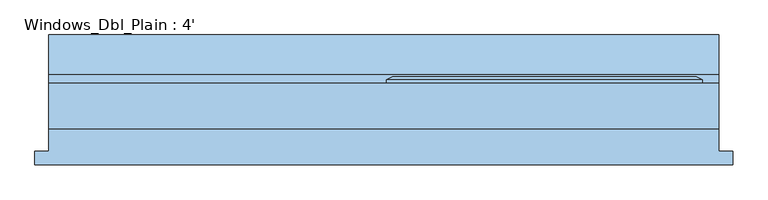
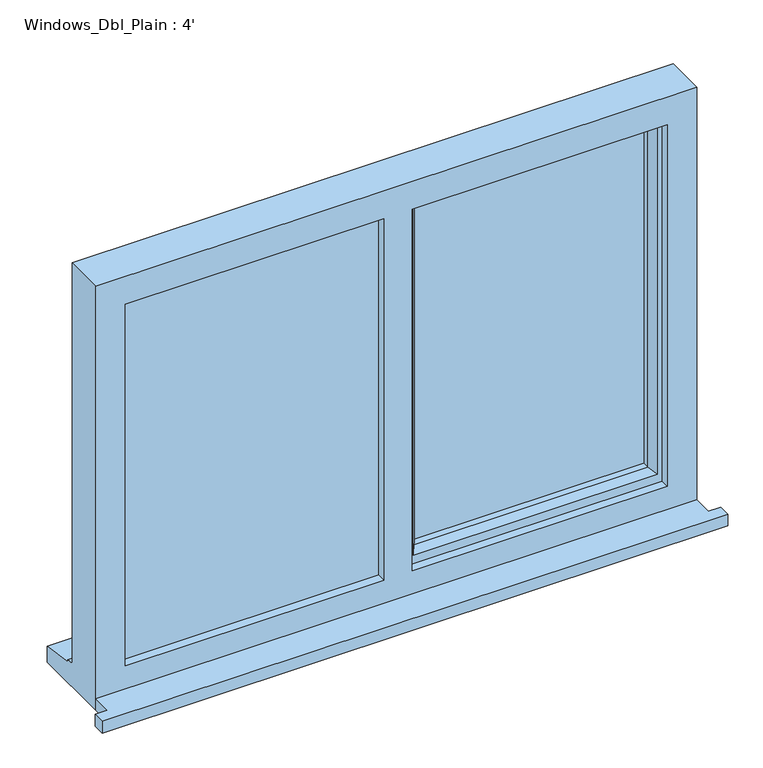
"""IFC4 building model written with IfcOpenShell, lengths in millimetres: window geometry, Windows_Dbl_Plain : 4'."""

from ifc_helpers import new_model, si_unit, frame, origin, place, context, project, spatial, polyline, outline, extrude, faceted_brep, source, transform, mapped, element, save


def windows_dbl_plain_4_44133fe2(model_context):
    return source(origin(), model_context, "Body", "SolidModel", [
        extrude(outline(polyline([(-919.6, -103.4114322), (-919.6, -78.4114322), (-894.6, -78.4114322), (-894.6, -37.6754322), (324.6, -37.6754322), (324.6, -78.4114322), (349.6, -78.4114322), (349.6, -103.4114322), (-919.6, -103.4114322)])), frame((0.0, 0.0, 1200.0), z_axis=(0.0, 0.0, 1.0), x_axis=(1.0, 0.0, 0.0)), (0.0, 0.0, 1.0), 25.0),
        faceted_brep([(-280.0, 45.3245678, 2080.0), (-280.0, 51.0980705, 2080.0), (-280.0, 51.0980705, 1253.0), (-280.0, 45.3245678, 1253.0), (-270.0, -19.6754322, 2070.0), (-270.0, 45.3245678, 2070.0), (-270.0, 45.3245678, 1263.0), (-270.0, -19.6754322, 1263.0), (-230.0, -5.1825323, 2030.0), (-240.1480377, -19.6754322, 2040.1480377), (-240.1480377, -19.6754322, 1292.8519623), (-230.0, -5.1825323, 1303.0), (-230.0, 9.3245678, 2030.0), (-230.0, 9.3245678, 1303.0), (-240.0, 33.3245678, 2040.0), (-240.0, 9.3245678, 2040.0), (-240.0, 9.3245678, 1293.0), (-240.0, 33.3245678, 1293.0), (-230.0, 51.0980705, 2030.0), (-230.0, 33.3245678, 2030.0), (-230.0, 33.3245678, 1303.0), (-230.0, 51.0980705, 1303.0), (-247.4457548, 56.8715732, 2047.4457548), (-247.4457548, 56.8715732, 1285.5542452), (-269.2153903, 56.8715732, 2069.2153903), (-269.2153903, 56.8715732, 1263.7846097), (294.6, 51.0980705, 1253.0), (294.6, 45.3245678, 1253.0), (284.6, 45.3245678, 1263.0), (284.6, -19.6754322, 1263.0), (254.7480377, -19.6754322, 1292.8519623), (244.6, -5.1825323, 1303.0), (244.6, 9.3245678, 1303.0), (254.6, 9.3245678, 1293.0), (254.6, 33.3245678, 1293.0), (244.6, 33.3245678, 1303.0), (244.6, 51.0980705, 1303.0), (262.0457548, 56.8715732, 1285.5542452), (283.8153903, 56.8715732, 1263.7846097), (294.6, 51.0980705, 2080.0), (294.6, 45.3245678, 2080.0), (284.6, 45.3245678, 2070.0), (284.6, -19.6754322, 2070.0), (254.7480377, -19.6754322, 2040.1480377), (244.6, -5.1825323, 2030.0), (244.6, 9.3245678, 2030.0), (254.6, 9.3245678, 2040.0), (254.6, 33.3245678, 2040.0), (244.6, 33.3245678, 2030.0), (244.6, 51.0980705, 2030.0), (262.0457548, 56.8715732, 2047.4457548), (283.8153903, 56.8715732, 2069.2153903)], [[[0, 1, 2, 3]], [[4, 5, 6, 7]], [[8, 9, 10, 11]], [[12, 8, 11, 13]], [[14, 15, 16, 17]], [[18, 19, 20, 21]], [[22, 18, 21, 23]], [[1, 24, 25, 2]], [[3, 2, 26, 27]], [[7, 6, 28, 29]], [[11, 10, 30, 31]], [[13, 11, 31, 32]], [[17, 16, 33, 34]], [[21, 20, 35, 36]], [[23, 21, 36, 37]], [[2, 25, 38, 26]], [[27, 26, 39, 40]], [[29, 28, 41, 42]], [[31, 30, 43, 44]], [[32, 31, 44, 45]], [[34, 33, 46, 47]], [[36, 35, 48, 49]], [[37, 36, 49, 50]], [[26, 38, 51, 39]], [[40, 39, 1, 0]], [[3, 27, 40, 0], [5, 41, 28, 6]], [[42, 41, 5, 4]], [[7, 29, 42, 4], [9, 43, 30, 10]], [[44, 43, 9, 8]], [[45, 44, 8, 12]], [[15, 46, 33, 16], [13, 32, 45, 12]], [[47, 46, 15, 14]], [[17, 34, 47, 14], [19, 48, 35, 20]], [[49, 48, 19, 18]], [[50, 49, 18, 22]], [[24, 51, 38, 25], [23, 37, 50, 22]], [[39, 51, 24, 1]]]),
        extrude(outline(polyline([(2050.0, -310.0), (2070.0, -310.0), (2070.0, -854.6), (1263.0, -854.6), (1263.0, -310.0), (1283.0, -310.0), (1283.0, -834.6), (2050.0, -834.6), (2050.0, -310.0)])), frame((0.0, 4.3245678, 0.0), z_axis=(0.0, 1.0, 0.0), x_axis=(0.0, 0.0, 1.0)), (0.0, 0.0, 1.0), 41.0),
        faceted_brep([(324.6, -37.6754322, 2110.0), (-894.6, -37.6754322, 2110.0), (-894.6, -37.6754322, 1200.0), (324.6, -37.6754322, 1200.0), (264.6, -37.6754322, 2050.0), (264.6, -37.6754322, 1275.0), (-252.0, -37.6754322, 1275.0), (-252.0, -37.6754322, 2050.0), (-310.0, -37.6754322, 2050.0), (-310.0, -37.6754322, 1275.0), (-834.6, -37.6754322, 1275.0), (-834.6, -37.6754322, 2050.0), (-894.6, 45.3245678, 2110.0), (-894.6, 45.3245678, 1251.0), (-894.6, 60.3245678, 1249.68767), (-894.6, 60.3245678, 1244.7449676), (-894.6, 132.8245678, 1233.8088847), (-894.6, 132.8245678, 1200.0), (324.6, 45.3245678, 2110.0), (324.6, 45.3245678, 1251.0), (-854.6, 45.3245678, 2070.0), (-854.6, 45.3245678, 1263.0), (-310.0, 45.3245678, 1263.0), (-310.0, 45.3245678, 2070.0), (-270.0, 45.3245678, 2070.0), (-270.0, 45.3245678, 1263.0), (284.6, 45.3245678, 1263.0), (284.6, 45.3245678, 2070.0), (-854.6, -19.6754322, 2070.0), (-854.6, -19.6754322, 1263.0), (-300.0, -19.6754322, 2070.0), (-300.0, -19.6754322, 1263.0), (-310.0, -19.6754322, 2050.0), (-834.6, -19.6754322, 2050.0), (-834.6, -19.6754322, 1275.0), (-310.0, -19.6754322, 1275.0), (-270.0, -19.6754322, 2070.0), (284.6, -19.6754322, 2070.0), (284.6, -19.6754322, 1263.0), (-270.0, -19.6754322, 1263.0), (264.6, -19.6754322, 2050.0), (-252.0, -19.6754322, 2050.0), (-252.0, -19.6754322, 1275.0), (264.6, -19.6754322, 1275.0), (-310.0, 4.3245678, 2070.0), (-300.0, 4.3245678, 2070.0), (324.6, 132.8245678, 1200.0), (324.6, 132.8245678, 1233.8088847), (324.6, 60.3245678, 1244.7449676), (324.6, 60.3245678, 1249.68767), (-300.0, 4.3245678, 1263.0), (-310.0, 4.3245678, 1263.0)], [[[0, 1, 2, 3], [4, 5, 6, 7], [8, 9, 10, 11]], [[2, 1, 12, 13, 14, 15, 16, 17]], [[13, 12, 18, 19], [20, 21, 22, 23], [24, 25, 26, 27]], [[21, 20, 28, 29]], [[28, 30, 31, 29], [32, 33, 34, 35]], [[36, 37, 38, 39], [40, 41, 42, 43]], [[33, 11, 10, 34]], [[1, 0, 18, 12]], [[28, 20, 23, 44, 45, 30]], [[27, 37, 36, 24]], [[11, 33, 32, 8]], [[40, 4, 7, 41]], [[19, 18, 0, 3, 46, 47, 48, 49]], [[27, 26, 38, 37]], [[4, 40, 43, 5]], [[45, 50, 31, 30]], [[50, 45, 44, 51]], [[51, 44, 23, 22]], [[25, 24, 36, 39]], [[41, 7, 6, 42]], [[8, 32, 35, 9]], [[46, 3, 2, 17]], [[47, 46, 17, 16]], [[48, 47, 16, 15]], [[49, 48, 15, 14]], [[19, 49, 14, 13]], [[22, 21, 29, 31, 50, 51]], [[26, 25, 39, 38]], [[6, 5, 43, 42]], [[35, 34, 10, 9]]]),
        extrude(outline(polyline([(-854.6, 4.3245678), (-300.0, 4.3245678), (-300.0, -19.6754322), (-854.6, -19.6754322), (-854.6, 4.3245678)])), frame((0.0, 0.0, 1263.0), z_axis=(0.0, 0.0, 1.0), x_axis=(1.0, 0.0, 0.0)), (0.0, 0.0, 1.0), 807.0),
        extrude(outline(polyline([(254.6, 9.3245678), (-240.0, 9.3245678), (-240.0, 33.3245678), (254.6, 33.3245678), (254.6, 9.3245678)])), frame((0.0, 0.0, 1293.0), z_axis=(0.0, 0.0, 1.0), x_axis=(1.0, 0.0, 0.0)), (0.0, 0.0, 1.0), 747.0),
    ])


if __name__ == "__main__":
    model = new_model("IFC4")
    model_context = context("Model", 3, world=origin())
    ifc_project = project(units=[si_unit("LENGTHUNIT", "METRE", prefix="MILLI")], contexts=[model_context])
    site = spatial("IfcSite", under=ifc_project)
    building = spatial("IfcBuilding", under=site)
    placement = place(None, origin())
    windows_dbl_plain_4_shape = windows_dbl_plain_4_44133fe2(model_context)
    element("IfcWindow", 1, ObjectType="Windows_Dbl_Plain : 4'", at=placement, inside=building, context=model_context, shape_type="MappedRepresentation", body=[
        mapped(windows_dbl_plain_4_shape, transform((0.0, 0.0, 0.0), x_axis=(1.0, 0.0, 0.0), y_axis=(0.0, 1.0, 0.0), z_axis=(0.0, 0.0, 1.0))),
    ])
    save(model, "model.ifc")

# Revit data of these elements
# Type "Windows_Dbl_Plain : 4'"
#   Type Mark = "56"
#   Operation = "DoublePanelVertical"
#   Construction Type Id = "GSP4R"
#   Manufacturer = "Revit"
#   Keynote = "L10"
#   Analytic Construction = "1/8 in Pilkington single glazing"
#   Wrap Layers (Ext) from Ext = 0.336286 ft
#   Wrap Layers (Int) from Ext = 0.582349 ft
#   Window Board Projection = 0.082021 ft
#   Window Board Extension = 0.082021 ft
#   Visual Light Transmittance = 0.9
#   Solar Heat Gain Coefficient = 0.78
#   Rough Width = 4.0 ft
#   Rough Height = 2.985564 ft
#   Height = 2.985564 ft
#   Width = 4.0 ft
#   Heat Transfer Coefficient (U) = 3.6886 W/(m²·K)
#   Glazing Thickness = 0.07874 ft
#   FrameOffset - External = 0.164042 ft
#   Frame Depth = 0.213255 ft
#   Default Head Height = 6.922572 ft
#   Cill Depth = 0.287073 ft
#   Cavity Closer Width = 0.164042 ft
#   Cavity Closer Offset from Ext = 0.336286 ft
#   Cavity Closer Depth = 0.278871 ft
#   Vis - Cavity Closers = yes
#   Define Thermal Properties by = 1
#   Material Trim = Window Frame
#   Material Glass = Glass
#   Material Frame = Window Frame
#   Wall Closure = (empty or 0)
# Element 1 (IfcWindow, "Windows_Dbl_Plain : 4'")
#   Materials on its faces: "Window Frame", "Glass"
# Materials
#   "Window Frame": colour RGB 249 249 249, transparency 0, Keynote = "L10", Cost = 0
#   "Glass": class "Glass", colour RGB 0 128 192, transparency 0.9, Description = "Soda Lime Glass", Cost = 0
